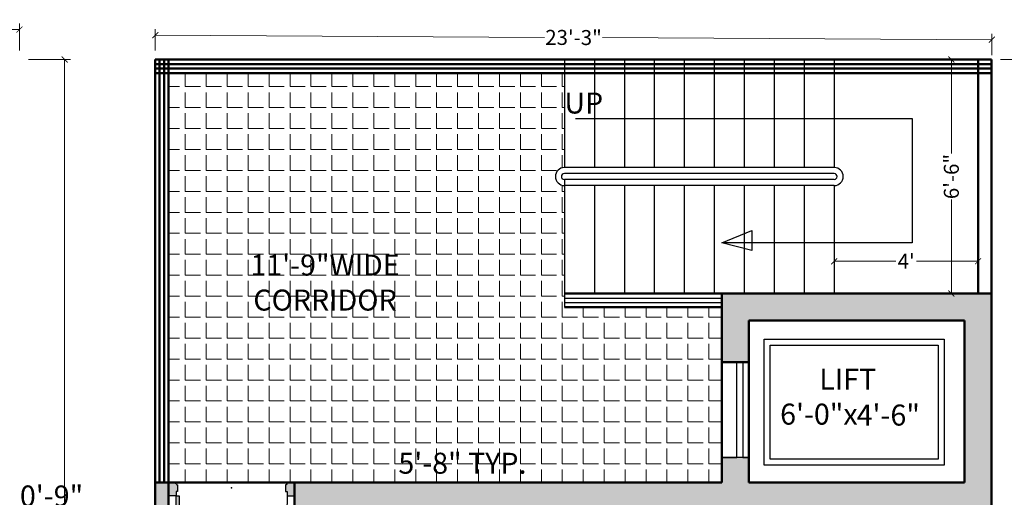
# Model space of a CAD drawing. Units: inches. Extents: x 4508 to 5907, y 877 to 1592.
# Tile 6 of 20: x 4874 to 5203, y 1429 to 1588. Entities that reach past the tile are written whole.
import ezdxf

# ---------------------------------------------------------------- set-up
doc = ezdxf.new("R2010")
doc.units = ezdxf.units.IN
doc.layers.get('DEFPOINTS').update_dxf_attribs({"color": 8})
for name, color, linetype, lineweight in [('A-ANNO-DIMS', 2, 'Continuous', 18), ('A-ANNO-TEXT', 7, 'Continuous', 25), ('A-DOOR', 4, 'Continuous', 25), ('A-EQPM', 6, 'Continuous', 25), ('A-FLOR-PATT', 252, 'Continuous', 13), ('A-FLOR-STRS', 5, 'Continuous', 25), ('A-WALL', 7, 'Continuous', 50), ('A-WALL-PATT', 8, 'Continuous', 13)]:
    doc.layers.add(name, color=color, linetype=linetype, lineweight=lineweight)
doc.layers.add('doors & windows', color=30, linetype='Continuous')
doc.styles.get("Standard").update_dxf_attribs({"font": 'arial.ttf'})
doc.dimstyles.new('details', dxfattribs={"dimtxt": 5, "dimasz": 2, "dimexe": 2, "dimexo": 3, "dimgap": 1, "dimtad": 0, "dimdec": 1, "dimzin": 0, "dimdsep": 46, "dimlunit": 4, "dimtxsty": 'Standard', "dimblk": 'ARCHTICK', "dimcen": 3, "dimclrd": 256, "dimclre": 256, "dimclrt": 256, "dimadec": 0, "dimazin": 0, "dimtfac": 0.5, "dimtdec": 1, "dimtofl": 0, "dimtmove": 0, "dimatfit": 3, "dimldrblk": 'CLOSEDBLANK', "dimfxl": 2, "dimtolj": 1, "dimtzin": 0, "dimlwd": -1, "dimlwe": -1, "dimarcsym": 0})
doc.dimstyles.new('text', dxfattribs={"dimtxt": 7, "dimasz": 0, "dimexe": 3, "dimexo": 3, "dimgap": 0, "dimtad": 1, "dimtih": 1, "dimtoh": 1, "dimzin": 3, "dimdsep": 46, "dimlunit": 4, "dimtxsty": 'Standard', "dimblk": 'CLOSEDBLANK', "dimcen": 3, "dimse1": 1, "dimse2": 1, "dimsd1": 1, "dimsd2": 1, "dimclrd": 256, "dimclre": 256, "dimclrt": 256, "dimadec": 0, "dimazin": 0, "dimtfac": 0.5, "dimtofl": 0, "dimtmove": 0, "dimatfit": 3, "dimfxl": 3, "dimtolj": 1, "dimtzin": 0, "dimlwd": -1, "dimlwe": -1, "dimarcsym": 0})

# ---------------------------------------------------------------- blocks, each defined once
blk = doc.blocks.new('_ArchTick')
at = {"color": 0, "linetype": 'ByBlock', "const_width": 0.15}
blk.add_lwpolyline([(-0.5, -0.5), (0.5, 0.5)], dxfattribs=at)
blk = doc.blocks.new('*D51')
at = {"layer": 'A-ANNO-DIMS', "color": 0, "transparency": 16777216}
for p, q in [((4595.24, 1577.7), (4595.24, 1586.7)), ((4874.24, 1577.7), (4874.24, 1586.7)), ((4595.24, 1584.7), (4725.11, 1584.7)), ((4874.24, 1584.7), (4744.37, 1584.7))]:
    blk.add_line(p, q, dxfattribs=at)
at = {"layer": 'DEFPOINTS', "color": 0, "transparency": 16777216}
for p in [(4874.24, 1584.7), (4595.24, 1574.7), (4874.24, 1574.7)]:
    blk.add_point(p, dxfattribs=at)
at = {"layer": 'A-ANNO-DIMS', "color": 0, "transparency": 16777216, "xscale": 2, "yscale": 2, "zscale": 2, "rotation": 180}
blk.add_blockref('_ArchTick', (4595.24, 1584.7), dxfattribs=at)
at = {"layer": 'A-ANNO-DIMS', "color": 0, "transparency": 16777216, "xscale": 2, "yscale": 2, "zscale": 2}
blk.add_blockref('_ArchTick', (4874.24, 1584.7), dxfattribs=at)
at = {"layer": 'A-ANNO-DIMS', "color": 0, "transparency": 16777216, "insert": (4734.74, 1584.7), "char_height": 5, "attachment_point": 5}
blk.add_mtext('\\A1;23\'-3"', dxfattribs=at)
blk = doc.blocks.new('_ClosedBlank')
at = {"color": 0, "lineweight": -2}
for p, q in [((-1, 0.17), (0, 0)), ((-1, 0.17), (-1, -0.17)), ((0, 0), (-1, -0.17))]:
    blk.add_line(p, q, dxfattribs=at)
blk = doc.blocks.new('*D52')
at = {"layer": 'A-ANNO-DIMS', "color": 0, "transparency": 16777216}
for p, q in [((4877.24, 1574.7), (4891.29, 1574.7)), ((4889.29, 1574.7), (4889.29, 1255.95)), ((4889.29, 926.7), (4889.29, 1245.46)), ((4877.24, 926.7), (4891.29, 926.7))]:
    blk.add_line(p, q, dxfattribs=at)
at = {"layer": 'DEFPOINTS', "color": 0, "transparency": 16777216}
for p in [(4874.24, 1574.7), (4874.24, 926.7), (4889.29, 926.7)]:
    blk.add_point(p, dxfattribs=at)
at = {"layer": 'A-ANNO-DIMS', "color": 0, "transparency": 16777216, "xscale": 2, "yscale": 2, "zscale": 2}
for p, rotation in [((4889.29, 1574.7), 90), ((4889.29, 926.7), 270)]:
    blk.add_blockref('_ArchTick', p, dxfattribs=dict(at, rotation=rotation))
at = {"layer": 'A-ANNO-DIMS', "color": 0, "transparency": 16777216, "insert": (4889.29, 1250.7), "char_height": 5, "attachment_point": 5, "rotation": 90}
blk.add_mtext("\\A1;54'", dxfattribs=at)
blk = doc.blocks.new('*D53')
at = {"layer": 'A-ANNO-DIMS', "color": 0, "transparency": 16777216}
for p, q in [((5190.99, 1574.7), (5183.06, 1574.7)), ((5185.06, 1574.7), (5185.06, 1543.36)), ((5185.06, 1496.7), (5185.06, 1528.04)), ((5190.99, 1496.7), (5183.06, 1496.7))]:
    blk.add_line(p, q, dxfattribs=at)
at = {"layer": 'DEFPOINTS', "color": 0, "transparency": 16777216}
for p in [(5185.06, 1574.7), (5193.99, 1574.7), (5193.99, 1496.7)]:
    blk.add_point(p, dxfattribs=at)
at = {"layer": 'A-ANNO-DIMS', "color": 0, "transparency": 16777216, "xscale": 2, "yscale": 2, "zscale": 2}
for p, rotation in [((5185.06, 1574.7), 90), ((5185.06, 1496.7), 270)]:
    blk.add_blockref('_ArchTick', p, dxfattribs=dict(at, rotation=rotation))
at = {"layer": 'A-ANNO-DIMS', "color": 0, "transparency": 16777216, "insert": (5185.06, 1535.7), "char_height": 5, "attachment_point": 5, "rotation": 90}
blk.add_mtext('\\A1;6\'-6"', dxfattribs=at)
blk = doc.blocks.new('*D54')
at = {"layer": 'A-ANNO-DIMS', "color": 0, "transparency": 16777216}
for p, q in [((5145.99, 1499.7), (5145.99, 1509.46)), ((5145.99, 1507.46), (5166.59, 1507.46)), ((5193.99, 1507.46), (5173.39, 1507.46)), ((5193.99, 1499.7), (5193.99, 1509.46))]:
    blk.add_line(p, q, dxfattribs=at)
at = {"layer": 'DEFPOINTS', "color": 0, "transparency": 16777216}
for p in [(5145.99, 1507.46), (5145.99, 1496.7), (5193.99, 1496.7)]:
    blk.add_point(p, dxfattribs=at)
at = {"layer": 'A-ANNO-DIMS', "color": 0, "transparency": 16777216, "xscale": 2, "yscale": 2, "zscale": 2, "rotation": 180}
blk.add_blockref('_ArchTick', (5145.99, 1507.46), dxfattribs=at)
at = {"layer": 'A-ANNO-DIMS', "color": 0, "transparency": 16777216, "xscale": 2, "yscale": 2, "zscale": 2}
blk.add_blockref('_ArchTick', (5193.99, 1507.46), dxfattribs=at)
at = {"layer": 'A-ANNO-DIMS', "color": 0, "transparency": 16777216, "insert": (5169.99, 1507.46), "char_height": 5, "attachment_point": 5}
blk.add_mtext("\\A1;4'", dxfattribs=at)
blk = doc.blocks.new('MD')
at = {"layer": 'doors & windows'}
h = blk.add_hatch(dxfattribs=at)
h.set_pattern_fill('DOTS', color=256, scale=2, style=0)
h.set_pattern_definition([(180, (0, -4), (-0.0625, 0.125), [0, -0.125])])
h.paths.add_polyline_path([(2.5, 37), (3.5, 37), (3.5, 0), (2.5, 0)])
h = blk.add_hatch(dxfattribs=at)
h.set_pattern_fill('DOTS', color=256, scale=2, style=0)
h.set_pattern_definition([(0, (0, -0.5), (0.0625, 0.125), [0, -0.125])])
h.paths.add_polyline_path([(42, -4.5), (42, 0), (39.5, 0), (39.5, -1.5), (39, -1.5), (39, -3.75), (39.25, -3.75, 0.403966), (39.75, -4.25), (39.75, -4.5)])
h.paths.add_polyline_path([(0, -4.5), (2.25, -4.5), (2.25, -4.25, 0.403966), (2.75, -3.75), (3, -3.75), (3, -1.5), (2.5, -1.5), (2.5, 0), (0, 0)])
for p, q in [((0, 0), (0, -4.5)), ((42, 0), (42, -4.5))]:
    blk.add_line(p, q)
blk.add_line((0, -4.5), (2.25, -4.5), dxfattribs=at)
blk.add_lwpolyline([(3.5, 0), (3.5, 37), (2.5, 37), (2.5, 0)], close=True, dxfattribs=at)
for points in [[(3, -3.75), (3, -1.5), (2.5, -1.5), (2.5, 0), (0, 0)], [(39, -3.75), (39, -1.5), (39.5, -1.5), (39.5, 0), (42, 0)], [(42, -4.5), (39.75, -4.5)]]:
    blk.add_lwpolyline(points, dxfattribs=at)
for points in [[(2.25, -4.5), (2.25, -4.25, 0.403966), (2.75, -3.75), (3, -3.75)], [(39.75, -4.5), (39.75, -4.25, -0.403966), (39.25, -3.75), (39, -3.75)]]:
    blk.add_lwpolyline(points, format="xyb", dxfattribs=at)
at = {"layer": 'doors & windows', "ltscale": 6}
blk.add_arc((3.73, 1.23), 35.79, 358.0281, 91.9719, dxfattribs=at)
at = {"layer": 'doors & windows'}
blk.add_point((21, -2.75), dxfattribs=at)
blk = doc.blocks.new('*D61')
at = {"layer": 'DEFPOINTS', "color": 0, "transparency": 16777216}
for p in [(5117.27, 1458.96), (5189.27, 1453.88), (5189.27, 1452.91)]:
    blk.add_point(p, dxfattribs=at)
at = {"layer": 'A-ANNO-DIMS', "color": 0, "transparency": 16777216, "insert": (5140.88, 1462.32), "char_height": 7, "attachment_point": 5}
blk.add_mtext('\\A1;         LIFT\\P6\'-0"x', dxfattribs=at)
blk = doc.blocks.new('*D62')
at = {"layer": 'DEFPOINTS', "color": 0, "transparency": 16777216}
for p in [(5159.68, 1487.7), (5164.02, 1487.7), (5156.63, 1433.7)]:
    blk.add_point(p, dxfattribs=at)
at = {"layer": 'A-ANNO-DIMS', "color": 0, "transparency": 16777216, "insert": (5164.02, 1456.18), "char_height": 7, "attachment_point": 5}
blk.add_mtext('\\A1;4\'-6"', dxfattribs=at)
blk = doc.blocks.new('*D75')
at = {"layer": 'DEFPOINTS', "color": 0, "transparency": 16777216}
for p in [(4975.39, 1574.7), (4975.39, 1433.7), (4976.16, 1433.7)]:
    blk.add_point(p, dxfattribs=at)
at = {"layer": 'A-ANNO-DIMS', "color": 0, "transparency": 16777216, "insert": (4976.16, 1500.35), "char_height": 7, "attachment_point": 5}
blk.add_mtext('\\A1;11\'-9"WIDE \\PCORRIDOR', dxfattribs=at)
blk = doc.blocks.new('*D76')
at = {"layer": 'A-ANNO-DIMS', "color": 0, "transparency": 16777216}
for p, q in [((4919.51, 1577.7), (4919.55, 1584.8)), ((5198.51, 1576.2), (5198.55, 1583.3)), ((4919.54, 1582.8), (5049.4, 1582.1)), ((5198.54, 1581.3), (5068.67, 1582))]:
    blk.add_line(p, q, dxfattribs=at)
at = {"layer": 'DEFPOINTS', "color": 0, "transparency": 16777216}
for p in [(5198.54, 1581.3), (4919.49, 1574.7), (5198.49, 1573.2)]:
    blk.add_point(p, dxfattribs=at)
at = {"layer": 'A-ANNO-DIMS', "color": 0, "transparency": 16777216, "xscale": 2, "yscale": 2, "zscale": 2}
for p, rotation in [((4919.54, 1582.8), 179.6919611426001), ((5198.54, 1581.3), 359.6919611426002)]:
    blk.add_blockref('_ArchTick', p, dxfattribs=dict(at, rotation=rotation))
at = {"layer": 'A-ANNO-DIMS', "color": 0, "transparency": 16777216, "insert": (5059.04, 1582.05), "char_height": 5, "attachment_point": 5, "rotation": 359.692}
blk.add_mtext('\\A1;23\'-3"', dxfattribs=at)
blk = doc.blocks.new('*D77')
at = {"layer": 'A-ANNO-DIMS', "color": 0, "transparency": 16777216}
for p, q in [((5201.49, 1574.7), (5213.97, 1574.7)), ((5211.97, 1574.7), (5211.97, 1255.95)), ((5211.97, 926.7), (5211.97, 1245.46)), ((5201.49, 926.7), (5213.97, 926.7))]:
    blk.add_line(p, q, dxfattribs=at)
at = {"layer": 'DEFPOINTS', "color": 0, "transparency": 16777216}
for p in [(5198.49, 1574.7), (5211.97, 1574.7), (5198.49, 926.7)]:
    blk.add_point(p, dxfattribs=at)
at = {"layer": 'A-ANNO-DIMS', "color": 0, "transparency": 16777216, "xscale": 2, "yscale": 2, "zscale": 2}
for p, rotation in [((5211.97, 1574.7), 90), ((5211.97, 926.7), 270)]:
    blk.add_blockref('_ArchTick', p, dxfattribs=dict(at, rotation=rotation))
at = {"layer": 'A-ANNO-DIMS', "color": 0, "transparency": 16777216, "insert": (5211.97, 1250.7), "char_height": 5, "attachment_point": 5, "rotation": 90}
blk.add_mtext("\\A1;54'", dxfattribs=at)
blk = doc.blocks.new('*D171')
at = {"layer": 'DEFPOINTS', "color": 0, "transparency": 16777216}
for p in [(4987.99, 1436.55), (4987.99, 1424.7), (5055.99, 1424.7)]:
    blk.add_point(p, dxfattribs=at)
at = {"layer": 'A-ANNO-DIMS', "transparency": 16777216, "insert": (5021.99, 1440.13), "char_height": 7, "attachment_point": 5}
blk.add_mtext('\\A1;5\'-8" TYP.', dxfattribs=at)
blk = doc.blocks.new('*D185')
at = {"layer": 'DEFPOINTS', "color": 0, "transparency": 16777216}
for p in [(4884.941772, 1433.703772), (4923.991772, 1433.703772), (4923.991772, 1424.703772)]:
    blk.add_point(p, dxfattribs=at)
at = {"layer": 'A-ANNO-DIMS', "transparency": 16777216, "insert": (4884.941772, 1429.203772), "char_height": 7, "attachment_point": 5}
blk.add_mtext('\\A1;0\'-9"', dxfattribs=at)

msp = doc.modelspace()

# ---------------------------------------------------------------- hatches: boundary and pattern name
at = {"layer": 'A-FLOR-PATT'}
h = msp.add_hatch(dxfattribs=at)
h.set_pattern_fill('ANGLE', color=256)
h.set_pattern_definition([(0, (-707.3365, 14.9854), (0, 6.985), [5.08, -1.905]), (90, (-707.3365, 14.9854), (-6.985, 4e-16), [5.08, -1.905])])
h.paths.add_polyline_path([(5108.492, 1433.704), (5108.492, 1492.204), (5055.992, 1492.204), (5055.992, 1532.704, -1), (5055.992, 1538.704), (5055.992, 1570.204), (4923.992, 1570.204), (4923.992, 1496.704), (4923.992, 1433.704), (4926.242, 1433.704)])
h.paths.add_polyline_path([(4947.611, 1487.235), (5004.351, 1487.235), (5004.351, 1513.403), (4947.611, 1513.403)], flags=24)
at = {"layer": 'A-WALL-PATT'}
h = msp.add_hatch(color=256, dxfattribs=at)
h.dxf.hatch_style = 1
h.paths.add_polyline_path([(5198.492, 1496.704), (5108.492, 1496.704), (5108.492, 1473.841), (5117.492, 1473.841), (5117.492, 1487.704), (5189.492, 1487.704), (5189.492, 1433.704), (5117.492, 1433.704), (5117.492, 1442.024), (5115.492, 1442.024), (5108.492, 1442.024), (5108.492, 1433.704), (4965.992, 1433.704), (4965.992, 1424.704), (5144.492, 1424.704), (5144.492, 1376.919), (5148.992, 1376.919), (5148.992, 1424.704), (5198.492, 1424.704)])
h.paths.add_polyline_path([(5060.492, 1424.704), (5055.992, 1424.704), (5055.992, 1324.204), (5060.492, 1324.204)])
h = msp.add_hatch(color=256, dxfattribs=at)
h.dxf.hatch_style = 1
h.paths.add_polyline_path([(5198.492, 1328.704), (5148.992, 1328.704), (5148.992, 1340.919), (5144.492, 1340.919), (5144.492, 1328.704), (5130.194, 1328.704), (5130.194, 1324.204), (5163.992, 1324.204), (5163.992, 1184.704), (5105.492, 1184.704), (5105.492, 1180.124), (5109.992, 1180.124), (5109.992, 1180.204), (5193.992, 1180.204), (5193.992, 1115.704), (5109.992, 1115.704), (5109.992, 1123.704), (5109.992, 1150.124), (5105.492, 1150.124), (5105.492, 1115.704), (5096.492, 1115.704), (5096.492, 1111.204), (5193.992, 1111.204), (5193.992, 931.204), (5060.492, 931.204), (5060.492, 977.704), (5055.992, 977.704), (5055.992, 935.704), (5054.492, 935.704), (4983.992, 935.704), (4983.992, 1007.704), (4991.992, 1007.704), (5055.992, 1007.704), (5060.492, 1007.704), (5060.492, 1111.204), (5060.492, 1115.704), (5060.492, 1144.204), (5055.992, 1144.204), (5055.992, 1012.204), (4957.397, 1012.204), (4957.397, 1007.704), (4979.492, 1007.704), (4979.492, 926.704), (5198.492, 926.704)])
h.paths.add_polyline_path([(5193.992, 1184.704), (5168.492, 1184.704), (5168.492, 1324.204), (5193.992, 1324.204)], flags=16)
h.paths.add_polyline_path([(4923.992, 1180.204), (5055.992, 1180.204), (5055.992, 1144.204), (5060.492, 1144.204), (5060.492, 1184.704), (4923.992, 1184.704), (4923.992, 1424.704), (4923.992, 1433.704), (4919.492, 1433.704), (4919.492, 1007.704), (4957.397, 1007.704), (4957.397, 1012.204), (4923.992, 1012.204)])

# ---------------------------------------------------------------- linework, layer by layer
at = {"layer": 'A-EQPM'}
for points in [[(5122.632, 1481.483), (5182.632, 1481.483), (5182.632, 1439.483), (5122.632, 1439.483)], [(5124.632, 1479.483), (5180.632, 1479.483), (5180.632, 1441.483), (5124.632, 1441.483)]]:
    msp.add_lwpolyline(points, close=True, dxfattribs=at)
msp.add_lwpolyline([(5108.492, 1473.841), (5117.492, 1473.841), (5115.492, 1473.841), (5115.492, 1442.024), (5117.492, 1442.024), (5108.492, 1442.024), (5113.492, 1442.024), (5113.492, 1473.841)], dxfattribs=at)
at = {"layer": 'A-FLOR-STRS'}
for p, q in [((5055.992, 1574.704), (5055.992, 1538.704)), ((5065.992, 1574.704), (5065.992, 1538.704)), ((5075.992, 1574.704), (5075.992, 1538.704)), ((5085.992, 1574.704), (5085.992, 1538.704)), ((5095.992, 1574.704), (5095.992, 1538.704)), ((5105.992, 1574.704), (5105.992, 1538.704)), ((5115.992, 1574.704), (5115.992, 1538.704)), ((5125.992, 1574.704), (5125.992, 1538.704)), ((5135.992, 1574.704), (5135.992, 1538.704)), ((5145.992, 1574.704), (5145.992, 1538.704)), ((5145.992, 1538.704), (5055.992, 1538.704)), ((5145.992, 1536.704), (5055.992, 1536.704)), ((5145.992, 1534.704), (5055.992, 1534.704)), ((5055.992, 1534.704), (5055.992, 1492.204)), ((5145.992, 1532.704), (5055.992, 1532.704)), ((5065.992, 1532.704), (5065.992, 1496.704)), ((5075.992, 1532.704), (5075.992, 1496.704)), ((5085.992, 1532.704), (5085.992, 1496.704)), ((5095.992, 1532.704), (5095.992, 1496.704)), ((5105.992, 1532.704), (5105.992, 1496.704)), ((5115.992, 1532.704), (5115.992, 1496.704)), ((5125.992, 1532.704), (5125.992, 1496.704)), ((5135.992, 1532.704), (5135.992, 1496.704)), ((5145.992, 1532.704), (5145.992, 1496.704)), ((5055.992, 1495.204), (5108.492, 1495.204)), ((5055.992, 1493.704), (5108.492, 1493.704))]:
    msp.add_line(p, q, dxfattribs=at)
msp.add_lwpolyline([(5059.657, 1555.099), (5171.987, 1555.099), (5171.987, 1513.599), (5108.49, 1513.599), (5118.49, 1517.728), (5118.49, 1511.051), (5108.49, 1513.599)], dxfattribs=at)
for centre, radius, start, end in [((5055.992, 1535.704), 3, 90, 270), ((5145.992, 1535.704), 3, 270, 90), ((5055.992, 1535.704), 1, 90, 270), ((5145.992, 1535.704), 1, 270, 90)]:
    msp.add_arc(centre, radius, start, end, dxfattribs=at)
at = {"layer": 'A-WALL'}
for p, q in [((4919.492, 1574.704), (5198.492, 1574.704)), ((4919.492, 926.704), (4919.492, 1574.704)), ((4919.492, 1573.204), (5198.492, 1573.204)), ((4920.992, 1433.704), (4920.992, 1574.704)), ((4922.492, 1433.704), (4922.492, 1574.704)), ((4923.992, 1496.704), (4923.992, 1574.704)), ((4923.992, 1424.704), (4923.992, 1574.704)), ((5193.992, 1574.704), (5193.992, 1496.704)), ((5198.492, 1574.704), (5198.492, 926.704)), ((4919.492, 1571.704), (5198.492, 1571.704)), ((4919.492, 1570.204), (5198.492, 1570.204)), ((5055.992, 1496.704), (5198.492, 1496.704)), ((5108.492, 1496.704), (5108.492, 1433.704)), ((5055.992, 1492.204), (5108.492, 1492.204)), ((5117.492, 1487.704), (5189.492, 1487.704)), ((5117.492, 1487.704), (5117.492, 1433.704)), ((5189.492, 1487.704), (5189.492, 1433.704)), ((5108.492, 1473.841), (5117.492, 1473.841)), ((5108.492, 1433.704), (4919.492, 1433.704)), ((4965.992, 1433.704), (4965.992, 1424.704)), ((5117.492, 1433.704), (5189.492, 1433.704))]:
    msp.add_line(p, q, dxfattribs=at)

# ---------------------------------------------------------------- block references
at = {"layer": 'A-DOOR', "xscale": -1, "rotation": 180}
msp.add_blockref('MD', (4923.992, 1429.204), dxfattribs=at)

# ---------------------------------------------------------------- texts
at = {"layer": 'A-ANNO-TEXT'}
msp.add_text('UP', height=7, dxfattribs=at).set_placement((5055.992, 1556.704))

# ---------------------------------------------------------------- dimensions: what is measured, and where the dimension line sits
at = {"layer": 'A-ANNO-DIMS'}
dim = msp.add_linear_dim(base=(4874.237, 1584.699), p1=(4595.237, 1574.704), p2=(4874.237, 1574.704), dimstyle='details', override={"dimclrd": 0, "dimclre": 0, "dimclrt": 0}, dxfattribs=at)
dim.commit()
dim.dimension.update_dxf_attribs({"geometry": '*D51', "text_midpoint": (4734.737, 1584.699)})
dim = msp.add_aligned_dim(p1=(4919.492, 1574.704), p2=(5198.492, 1573.204), distance=8.098, dimstyle='details', override={"dimclrd": 0, "dimclre": 0, "dimclrt": 0}, dxfattribs=at)
dim.commit()
dim.dimension.update_dxf_attribs({"geometry": '*D76', "text_midpoint": (5059.035, 1582.051)})
for base, p1, p2, dimstyle, override, picture, middle in [((4889.286, 926.704), (4874.237, 1574.704), (4874.237, 926.704), 'details', {"dimclrd": 0, "dimclre": 0, "dimclrt": 0}, '*D52', (4889.286, 1250.704)), ((5211.971, 1574.704), (5198.492, 926.704), (5198.492, 1574.704), 'details', {"dimclrd": 0, "dimclre": 0, "dimclrt": 0}, '*D77', (5211.971, 1250.704)), ((4884.942, 1433.704), (4923.992, 1424.704), (4923.992, 1433.704), 'text', {"dimdec": 1, "dimlfac": 1, "dimrnd": 0, "dimzin": 1, "dimdsep": 46, "dimlunit": 4, "dimfrac": 2}, '*D185', (4884.942, 1429.204))]:
    dim = msp.add_linear_dim(base=base, p1=p1, p2=p2, angle=90, dimstyle=dimstyle, override=override, dxfattribs=at)
    dim.commit()
    dim.dimension.update_dxf_attribs({"geometry": picture, "text_midpoint": middle})
dim = msp.add_linear_dim(base=(4976.162, 1433.704), p1=(4975.389, 1574.704), p2=(4975.389, 1433.704), angle=90, text='<>WIDE \\PCORRIDOR', dimstyle='text', override={"dimclrd": 0, "dimclre": 0, "dimclrt": 0}, dxfattribs=at)
dim.commit()
dim.dimension.update_dxf_attribs({"geometry": '*D75', "text_midpoint": (4976.162, 1500.345), "dimtype": 160})
for base, p1, p2, angle, dimstyle, picture, middle in [((5185.061, 1574.704), (5193.992, 1496.704), (5193.992, 1574.704), 90, 'details', '*D53', (5185.061, 1535.704)), ((5164.023, 1487.704), (5156.632, 1433.704), (5159.677, 1487.704), 270, 'text', '*D62', (5164.023, 1456.179))]:
    dim = msp.add_linear_dim(base=base, p1=p1, p2=p2, angle=angle, dimstyle=dimstyle, override={"dimclrd": 0, "dimclre": 0, "dimclrt": 0}, dxfattribs=at)
    dim.commit()
    dim.dimension.update_dxf_attribs({"geometry": picture, "text_midpoint": middle, "dimtype": 160})
dim = msp.add_linear_dim(base=(5145.992, 1507.459), p1=(5193.992, 1496.704), p2=(5145.992, 1496.704), dimstyle='details', override={"dimclrd": 0, "dimclre": 0, "dimclrt": 0}, dxfattribs=at)
dim.commit()
dim.dimension.update_dxf_attribs({"geometry": '*D54', "text_midpoint": (5169.992, 1507.459), "dimtype": 160})
dim = msp.add_linear_dim(base=(5189.267, 1452.914), p1=(5117.267, 1458.961), p2=(5189.267, 1453.877), text='         LIFT\\P<>x', dimstyle='text', override={"dimclrd": 0, "dimclre": 0, "dimclrt": 0}, dxfattribs=at)
dim.commit()
dim.dimension.update_dxf_attribs({"geometry": '*D61', "text_midpoint": (5140.88, 1452.914), "dimtype": 160})
dim = msp.add_linear_dim(base=(4987.992, 1436.554), p1=(5055.992, 1424.704), p2=(4987.992, 1424.704), angle=180, text='<> TYP.', dimstyle='text', override={"dimdec": 1, "dimrnd": 0, "dimzin": 1, "dimlunit": 4, "dimfrac": 2}, dxfattribs=at)
dim.commit()
dim.dimension.update_dxf_attribs({"geometry": '*D171', "text_midpoint": (5021.992, 1440.128)})

doc.saveas('drawing.dxf')
